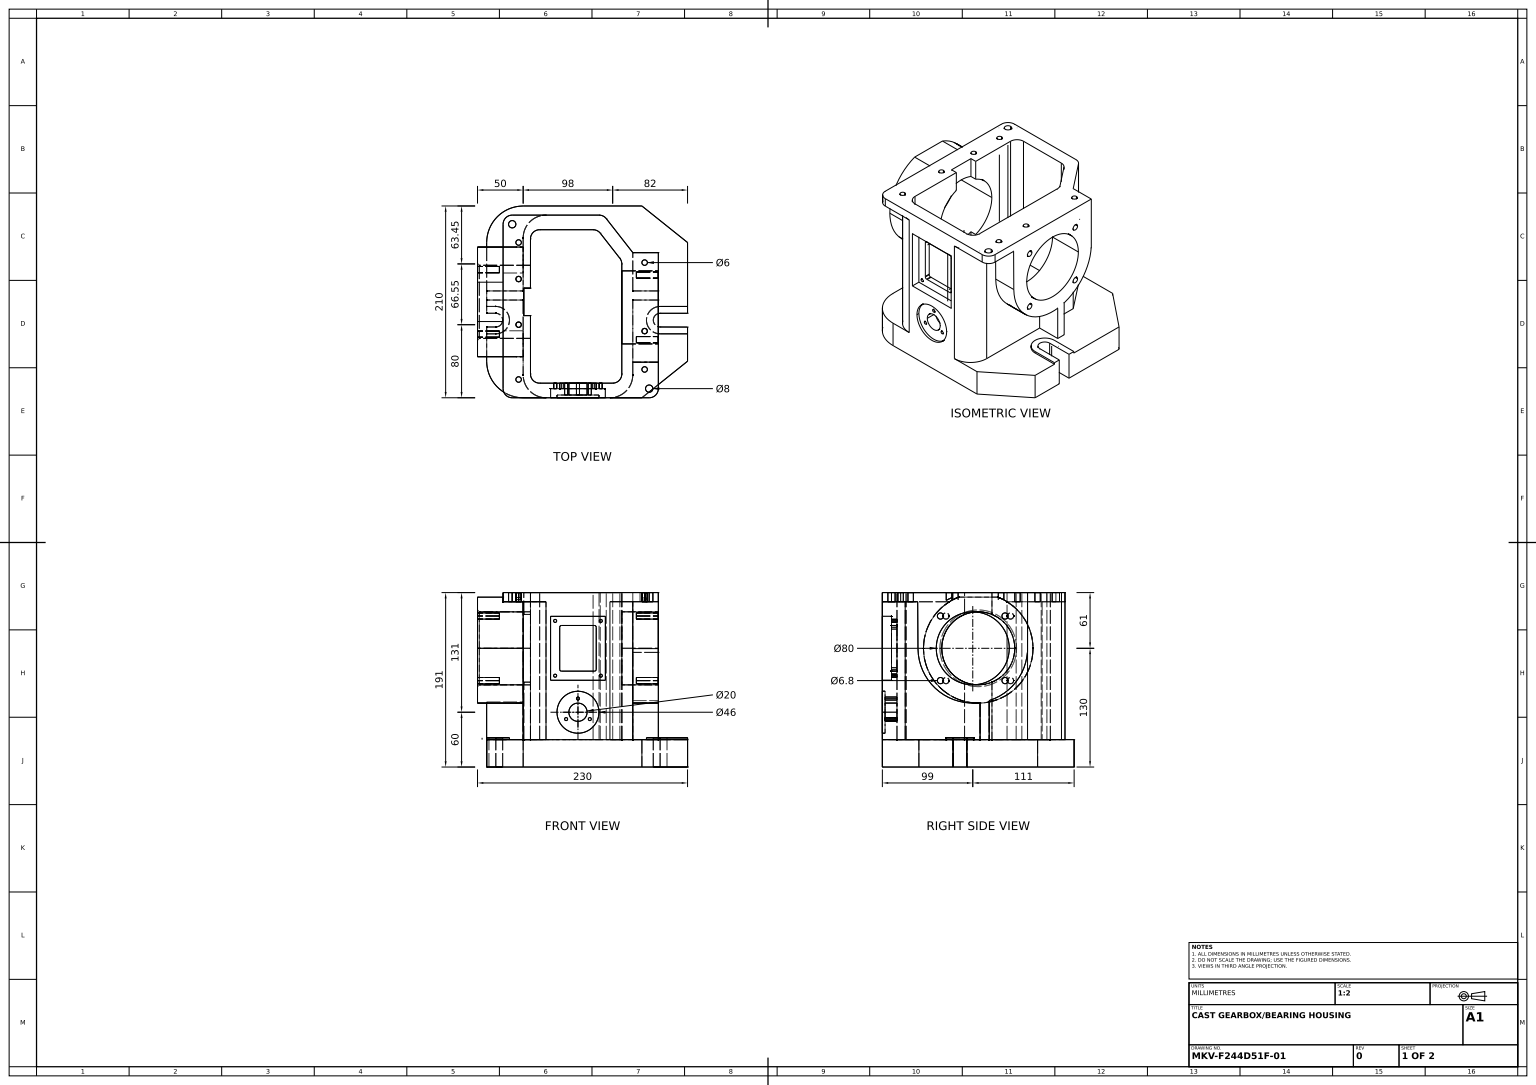
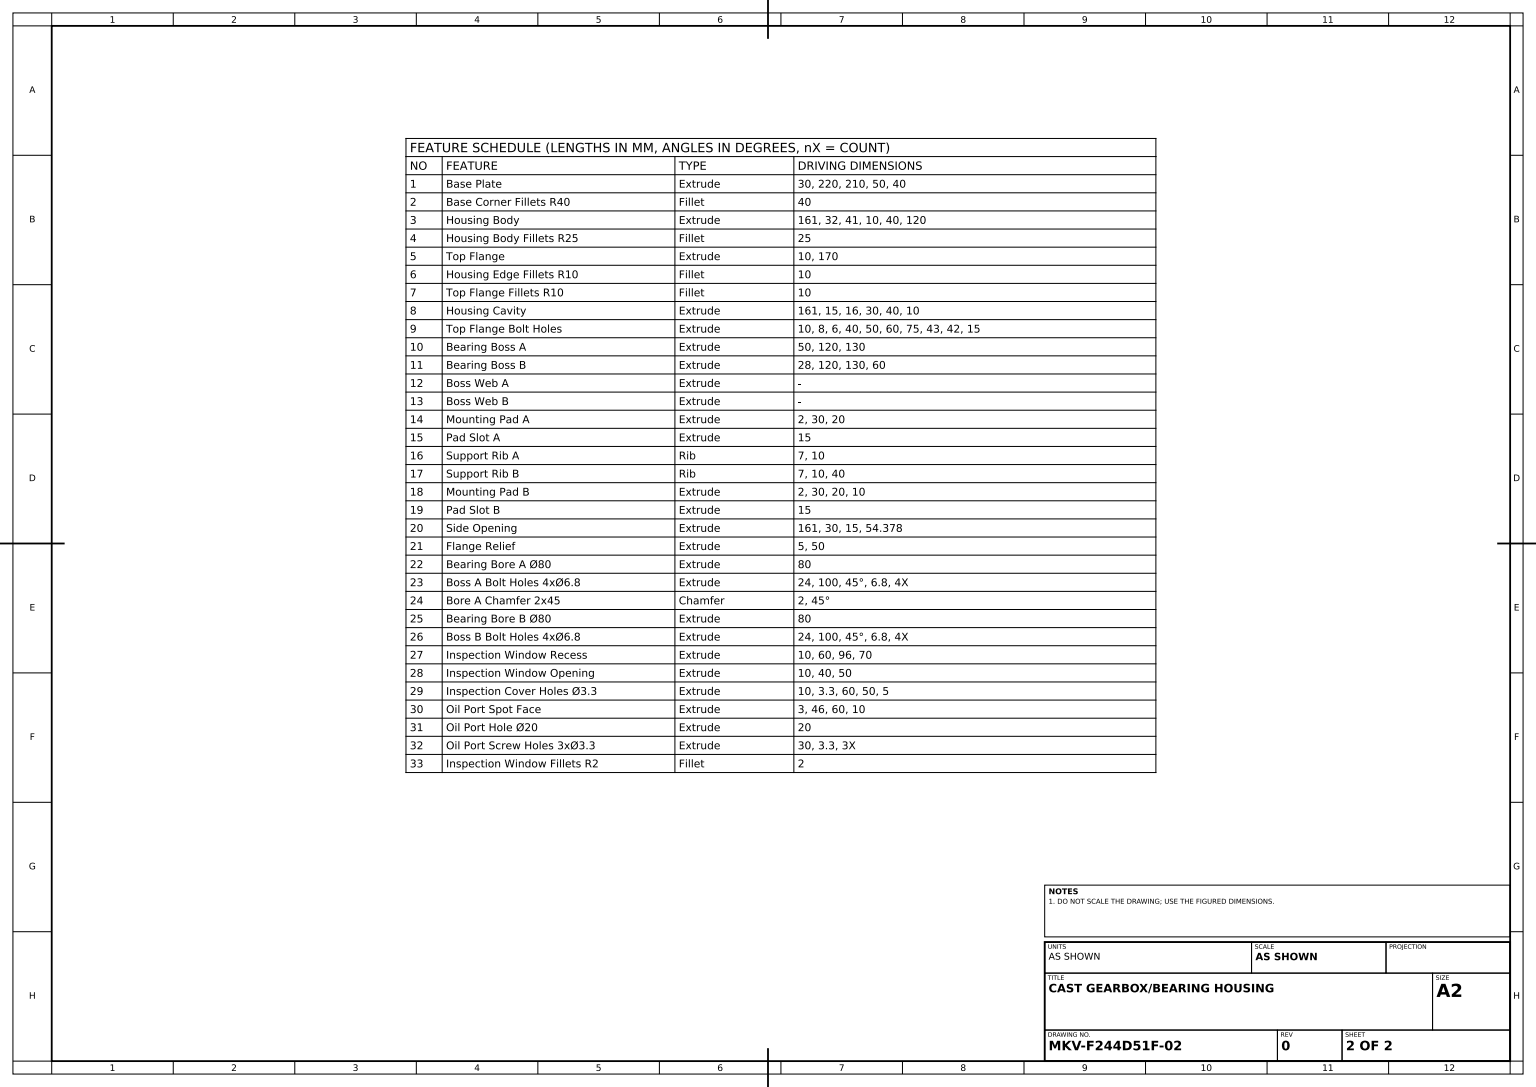
from build123d import *

# Parameters (mm, degrees)
BASE_PLATE_DEPTH                   = 30
BASE_CORNER_FILLETS_R40_R          = 40
HOUSING_BODY_DEPTH                 = 161
HOUSING_BODY_FILLETS_R25_R         = 25
TOP_FLANGE_DEPTH                   = 10
HOUSING_EDGE_FILLETS_R10_R         = 10
TOP_FLANGE_FILLETS_R10_R           = 10
HOUSING_CAVITY_DEPTH               = 161
TOP_FLANGE_BOLT_HOLES_SKETCH_R     = 4
TOP_FLANGE_BOLT_HOLES_SKETCH_R_2   = 3
TOP_FLANGE_BOLT_HOLES_DEPTH        = 10
BEARING_BOSS_A_SKETCH_R            = 60
BEARING_BOSS_A_DEPTH               = 50
BEARING_BOSS_B_SKETCH_R            = 60
BEARING_BOSS_B_DEPTH               = 28
BOSS_WEB_A_REACH                   = 277.975
BOSS_WEB_A_END_RADIUS              = 60
BOSS_WEB_A_SKETCH_W                = 28
BOSS_WEB_A_SKETCH_H                = 55.5
BOSS_WEB_B_REACH                   = 296.466
MOUNTING_PAD_A_DEPTH               = 2
PAD_SLOT_A_DEPTH                   = 226.179928128
SUPPORT_RIB_A_REACH                = 253.843
SUPPORT_RIB_A_SKETCH_WALL_W        = 545.68641053
SUPPORT_RIB_A_SKETCH_WALL_H        = 10
SUPPORT_RIB_B_REACH                = 253.843
SUPPORT_RIB_B_SKETCH_WALL_W        = 545.68641053
SUPPORT_RIB_B_SKETCH_WALL_H        = 10
MOUNTING_PAD_B_DEPTH               = 2
PAD_SLOT_B_DEPTH                   = 226.179928128
SIDE_OPENING_SKETCH_W              = 15
SIDE_OPENING_SKETCH_H              = 30
SIDE_OPENING_DEPTH                 = 161
FLANGE_RELIEF_SKETCH_W             = 28
FLANGE_RELIEF_SKETCH_H             = 50
FLANGE_RELIEF_DEPTH                = 5
BEARING_BORE_A_80_REACH            = 318.869
BEARING_BORE_A_SKETCH_R            = 40
BOSS_A_BOLT_HOLES_SKETCH_R         = 3.4
BOSS_A_BOLT_HOLES_4X_6_8_DEPTH     = 24
BORE_A_CHAMFER_2X45_SIZE           = 2
BEARING_BORE_B_80_REACH            = 296.466
BEARING_BORE_B_SKETCH_R            = 40
BOSS_B_BOLT_HOLES_SKETCH_R         = 3.4
BOSS_B_BOLT_HOLES_4X_6_8_DEPTH     = 24
INSPECTION_WINDOW_RECESS_SKETCH_W  = 60
INSPECTION_WINDOW_RECESS_SKETCH_H  = 70
INSPECTION_WINDOW_RECESS_DEPTH     = 10
INSPECTION_WINDOW_OPENING_SKETCH_W = 40
INSPECTION_WINDOW_OPENING_SKETCH_H = 50
INSPECTION_WINDOW_OPENING_DEPTH    = 10
INSPECTION_COVER_HOLES_SKETCH_R    = 1.65
INSPECTION_COVER_HOLES_3_3_DEPTH   = 10
OIL_PORT_SPOT_FACE_SKETCH_R        = 23
OIL_PORT_SPOT_FACE_DEPTH           = 3
OIL_PORT_HOLE_20_REACH             = 308.154
OIL_PORT_HOLE_SKETCH_R             = 10
OIL_PORT_SCREW_HOLES_3X_3_3_REACH  = 308.154
OIL_PORT_SCREW_HOLES_SKETCH_R      = 1.65
INSPECTION_WINDOW_FILLETS_R2_R     = 2


with BuildPart() as part:
    # Base Plate Sketch → Base Plate (new body)
    with BuildSketch(Plane(origin=(0, 0, 0), x_dir=(1, 0, 0), z_dir=(0, 1, 0))):
        Polygon((60, 105), (110, 65), (110, -65), (60, -105), (-110, -105), (-110, 105), align=None)
    extrude(amount=BASE_PLATE_DEPTH)

    # Base Corner Fillets R40
    base_corner_fillets_r40_edges = [part.edges().sort_by_distance(p)[0] for p in [
        (-110, 15, -105),
        (-110, 15, 105),
    ]]
    fillet(base_corner_fillets_r40_edges, radius=BASE_CORNER_FILLETS_R40_R)

    # Housing Body Sketch → Housing Body (add)
    with BuildSketch(Plane(origin=(0, 30, 0), x_dir=(1, 0, 0), z_dir=(0, 1, 0))):
        Polygon((-70, 95), (18, 95), (50, 54), (50, -105), (-70, -105), align=None)
    extrude(amount=HOUSING_BODY_DEPTH)

    # Housing Body Fillets R25
    housing_body_fillets_r25_edges = [part.edges().sort_by_distance(p)[0] for p in [
        (-70, 110.5, -95),
        (-70, 110.5, 105),
        (50, 110.5, 105),
    ]]
    fillet(housing_body_fillets_r25_edges, radius=HOUSING_BODY_FILLETS_R25_R)

    # Top Flange Sketch → Top Flange (add)
    with BuildSketch(Plane(origin=(0, 191, 0), x_dir=(1, 0, 0), z_dir=(0, 1, 0))):
        Polygon((18, 95), (-92, 95), (-92, -105), (78, -105), (78, 54), (50, 54), align=None)
    extrude(amount=-TOP_FLANGE_DEPTH)

    # Housing Edge Fillets R10
    housing_edge_fillets_r10_edges = [part.edges().sort_by_distance(p)[0] for p in [
        (18, 110.5, -95),
    ]]
    fillet(housing_edge_fillets_r10_edges, radius=HOUSING_EDGE_FILLETS_R10_R)

    # Top Flange Fillets R10
    top_flange_fillets_r10_edges = [part.edges().sort_by_distance(p)[0] for p in [
        (-92, 186, -95),
        (78, 186, 105),
        (-92, 186, 105),
    ]]
    fillet(top_flange_fillets_r10_edges, radius=TOP_FLANGE_FILLETS_R10_R)

    # Housing Cavity Sketch → Housing Cavity (cut)
    with BuildSketch(Plane(origin=(0, 191, 0), x_dir=(1, 0, 0), z_dir=(0, 1, 0))):
        with BuildLine():
            Line((35.883157835, 47.707697229), (14.462661191, 75.152708554))
            ThreePointArc((14.462661191, 75.152708554), (10.965441936, 77.986853886), (6.579503356, 79))
            Line((6.579503356, 79), (-52, 79))
            ThreePointArc((-52, 79), (-59.071067812, 76.071067812), (-62, 69))
            Line((-62, 69), (-62, -79))
            ThreePointArc((-62, -79), (-59.071067812, -86.071067812), (-52, -89))
            Line((-52, -89), (28, -89))
            ThreePointArc((28, -89), (35.071067812, -86.071067812), (38, -79))
            Line((38, -79), (38, 41.554988675))
            ThreePointArc((38, 41.554988675), (37.455992236, 44.808327088), (35.883157835, 47.707697229))
        make_face()
    extrude(amount=-HOUSING_CAVITY_DEPTH, mode=Mode.SUBTRACT)

    # Top Flange Bolt Holes Sketch → Top Flange Bolt Holes (cut)
    with BuildSketch(Plane(origin=(0, 191, 0), x_dir=(1, 0, 0), z_dir=(0, 1, 0))):
        with Locations(Location((-82, 85, 0), (0, 0, 270))):
            Circle(TOP_FLANGE_BOLT_HOLES_SKETCH_R)
        with Locations(Location((68, -95, 0), (0, 0, 270))):
            Circle(TOP_FLANGE_BOLT_HOLES_SKETCH_R)
        with Locations(Location((-75, 65, 0), (0, 0, 270))):
            Circle(TOP_FLANGE_BOLT_HOLES_SKETCH_R_2)
        with Locations(Location((-75, 25, 0), (0, 0, 270))):
            Circle(TOP_FLANGE_BOLT_HOLES_SKETCH_R_2)
        with Locations(Location((-75, -25, 0), (0, 0, 270))):
            Circle(TOP_FLANGE_BOLT_HOLES_SKETCH_R_2)
        with Locations(Location((-75, -85, 0), (0, 0, 270))):
            Circle(TOP_FLANGE_BOLT_HOLES_SKETCH_R_2)
        with Locations(Location((63, 43, 0), (0, 0, 270))):
            Circle(TOP_FLANGE_BOLT_HOLES_SKETCH_R_2)
        with Locations(Location((63, -32, 0), (0, 0, 270))):
            Circle(TOP_FLANGE_BOLT_HOLES_SKETCH_R_2)
        with Locations(Location((63, -74, 0), (0, 0, 270))):
            Circle(TOP_FLANGE_BOLT_HOLES_SKETCH_R_2)
    extrude(amount=-TOP_FLANGE_BOLT_HOLES_DEPTH, mode=Mode.SUBTRACT)

    # Bearing Boss A Sketch → Bearing Boss A (add)
    with BuildSketch(Plane.ZY.offset(70)):
        with Locations(Location((0, 130, 0), (0, 0, 121.788330617))):
            Circle(BEARING_BOSS_A_SKETCH_R)
    extrude(amount=BEARING_BOSS_A_DEPTH)

    # Bearing Boss B Sketch → Bearing Boss B (add)
    with BuildSketch(Plane(origin=(50, 0, 0), x_dir=(0, 0, -1), z_dir=(1, 0, 0))):
        with Locations((-6, 130)):
            Circle(BEARING_BOSS_B_SKETCH_R)
    extrude(amount=BEARING_BOSS_B_DEPTH)

    # Boss Web A: up to this cylinder (the profile starts outside it)
    boss_web_a_end = Plane(origin=(64, 130, 6), z_dir=(-1, 0, 0)) * Cylinder(BOSS_WEB_A_END_RADIUS, 676.95, mode=Mode.PRIVATE)
    # Boss Web A Sketch → Boss Web A (add, up to the surface)
    with BuildSketch(Plane(origin=(0, 0, -54), x_dir=(-1, 0, 0), z_dir=(0, 0, -1)), mode=Mode.PRIVATE) as boss_web_a_sk1:
        with Locations((-64, 153.25)):
            Rectangle(BOSS_WEB_A_SKETCH_W, BOSS_WEB_A_SKETCH_H)
    boss_web_a_tool1 = extrude(boss_web_a_sk1.sketch, amount=-BOSS_WEB_A_REACH, mode=Mode.PRIVATE) - boss_web_a_end
    add(boss_web_a_tool1.solids().sort_by_distance((64, 153.25, -54))[0])
    add(boss_web_a_tool1.solids().sort_by_distance((64, 153.25, -54))[1])

    # Boss Web B Sketch → Boss Web B (add, up to next)
    with BuildSketch(Plane(origin=(78, 0, 0), x_dir=(0, 0, -1), z_dir=(1, 0, 0)), mode=Mode.PRIVATE) as boss_web_b_sk1:
        with BuildLine():
            Line((-65.998945111, 129.644211289), (-66.303480629, 181))
            Line((-66.303480629, 181), (-37.606961259, 181))
            ThreePointArc((-37.606961259, 181), (-58.509663672, 159.029902188), (-65.998945111, 129.644211289))
        make_face()
    boss_web_b_tool1 = extrude(boss_web_b_sk1.sketch, amount=-BOSS_WEB_B_REACH, mode=Mode.PRIVATE) - part.part
    add(boss_web_b_tool1.solids().sort_by_distance((78, 168.840925, 58.135021))[0])

    # Mounting Pad A Sketch → Mounting Pad A (add)
    with BuildSketch(Plane(origin=(0, 30, 0), x_dir=(1, 0, 0), z_dir=(0, 1, 0))):
        with BuildLine():
            Line((80, -5), (110, -5))
            Line((110, -5), (110, -35))
            Line((110, -35), (80, -35))
            ThreePointArc((80, -35), (65, -20), (80, -5))
        make_face()
    extrude(amount=MOUNTING_PAD_A_DEPTH)

    # Pad Slot A Sketch → Pad Slot A (cut, through all)
    with BuildSketch(Plane(origin=(0, 32, 0), x_dir=(1, 0, 0), z_dir=(0, 1, 0))):
        with BuildLine():
            Line((80, -12.5), (110, -12.5))
            Line((110, -12.5), (110, -27.596191178))
            Line((110, -27.596191178), (79.975961959, -27.499961478))
            ThreePointArc((79.975961959, -27.499961478), (72.50000963, -19.987980964), (80, -12.5))
        make_face()
    extrude(amount=-PAD_SLOT_A_DEPTH, mode=Mode.SUBTRACT)

    # Support Rib A Sketch wall → Support Rib A (add, up to next)
    with BuildSketch(Plane(origin=(78, 50, -7), x_dir=(0, -1, 0), z_dir=(1, 0, 0)), mode=Mode.PRIVATE) as support_rib_a_sk1:
        Rectangle(SUPPORT_RIB_A_SKETCH_WALL_W, SUPPORT_RIB_A_SKETCH_WALL_H)
    support_rib_a_tool1 = extrude(support_rib_a_sk1.sketch, amount=-SUPPORT_RIB_A_REACH, mode=Mode.PRIVATE) - part.part
    add(support_rib_a_tool1.solids().sort_by_distance((78, 50, -7))[0])

    # Support Rib B Sketch wall → Support Rib B (add, up to next)
    with BuildSketch(Plane(origin=(-110, 50, -7), x_dir=(0, -1, 0), z_dir=(1, 0, 0)), mode=Mode.PRIVATE) as support_rib_b_sk1:
        Rectangle(SUPPORT_RIB_B_SKETCH_WALL_W, SUPPORT_RIB_B_SKETCH_WALL_H)
    support_rib_b_tool1 = extrude(support_rib_b_sk1.sketch, amount=SUPPORT_RIB_B_REACH, mode=Mode.PRIVATE) - part.part
    add(support_rib_b_tool1.solids().sort_by_distance((-110, 50, -7))[0])

    # Mounting Pad B Sketch → Mounting Pad B (add)
    with BuildSketch(Plane(origin=(0, 30, 0), x_dir=(1, 0, 0), z_dir=(0, 1, 0))):
        with BuildLine():
            Line((-100, -5), (-110, -5))
            Line((-110, -5), (-110, -35))
            Line((-110, -35), (-100, -35))
            ThreePointArc((-100, -35), (-85, -20), (-100, -5))
        make_face()
    extrude(amount=MOUNTING_PAD_B_DEPTH)

    # Pad Slot B Sketch → Pad Slot B (cut, through all)
    with BuildSketch(Plane(origin=(0, 32, 0), x_dir=(1, 0, 0), z_dir=(0, 1, 0))):
        with BuildLine():
            Line((-100, -12.5), (-110, -12.5))
            Line((-110, -12.5), (-110, -27.5))
            Line((-110, -27.5), (-100, -27.5))
            ThreePointArc((-100, -27.5), (-92.5, -20), (-100, -12.5))
        make_face()
    extrude(amount=-PAD_SLOT_B_DEPTH, mode=Mode.SUBTRACT)

    # Side Opening Sketch → Side Opening (cut)
    with BuildSketch(Plane(origin=(0, 191, 0), x_dir=(1, 0, 0), z_dir=(0, 1, 0))):
        with Locations((-61.877981693, 0)):
            Rectangle(SIDE_OPENING_SKETCH_W, SIDE_OPENING_SKETCH_H)
    extrude(amount=-SIDE_OPENING_DEPTH, mode=Mode.SUBTRACT)

    # Flange Relief Sketch → Flange Relief (cut)
    with BuildSketch(Plane(origin=(0, 191, 0), x_dir=(1, 0, 0), z_dir=(0, 1, 0))):
        with Locations((-106, 0)):
            Rectangle(FLANGE_RELIEF_SKETCH_W, FLANGE_RELIEF_SKETCH_H)
    extrude(amount=-FLANGE_RELIEF_DEPTH, mode=Mode.SUBTRACT)

    # Bearing Bore A Sketch → Bearing Bore A Ø80 (cut, up to next)
    with BuildSketch(Plane.ZY.offset(120), mode=Mode.PRIVATE) as bearing_bore_a_80_sk1:
        with Locations((0, 130)):
            Circle(BEARING_BORE_A_SKETCH_R)
    bearing_bore_a_80_tool1 = extrude(bearing_bore_a_80_sk1.sketch, amount=-BEARING_BORE_A_80_REACH, mode=Mode.PRIVATE) & part.part
    add(bearing_bore_a_80_tool1.solids().sort_by_distance((-120, 130, 0))[0], mode=Mode.SUBTRACT)

    # Boss A Bolt Holes Sketch → Boss A Bolt Holes 4xØ6.8 (cut)
    with BuildSketch(Plane.ZY.offset(120)):
        with Locations((35.355339059, 94.644660941)):
            Circle(BOSS_A_BOLT_HOLES_SKETCH_R)
        with Locations((-35.355339059, 94.644660941)):
            Circle(BOSS_A_BOLT_HOLES_SKETCH_R)
        with Locations((-35.355339059, 165.355339059)):
            Circle(BOSS_A_BOLT_HOLES_SKETCH_R)
        with Locations((35.355339059, 165.355339059)):
            Circle(BOSS_A_BOLT_HOLES_SKETCH_R)
    extrude(amount=-BOSS_A_BOLT_HOLES_4X_6_8_DEPTH, mode=Mode.SUBTRACT)

    # Bore A Chamfer 2x45
    bore_a_chamfer_2x45_edges = [part.edges().sort_by_distance(p)[0] for p in [
        (-120, 130, -40),
    ]]
    chamfer(bore_a_chamfer_2x45_edges, length=BORE_A_CHAMFER_2X45_SIZE)

    # Bearing Bore B Sketch → Bearing Bore B Ø80 (cut, up to next)
    with BuildSketch(Plane(origin=(78, 0, 0), x_dir=(0, 0, -1), z_dir=(1, 0, 0)), mode=Mode.PRIVATE) as bearing_bore_b_80_sk1:
        with Locations((-6, 130)):
            Circle(BEARING_BORE_B_SKETCH_R)
    bearing_bore_b_80_tool1 = extrude(bearing_bore_b_80_sk1.sketch, amount=-BEARING_BORE_B_80_REACH, mode=Mode.PRIVATE) & part.part
    add(bearing_bore_b_80_tool1.solids().sort_by_distance((78, 130, 6))[0], mode=Mode.SUBTRACT)

    # Boss B Bolt Holes Sketch → Boss B Bolt Holes 4xØ6.8 (cut)
    with BuildSketch(Plane(origin=(78, 0, 0), x_dir=(0, 0, -1), z_dir=(1, 0, 0))):
        with Locations((29.355339059, 94.644660941)):
            Circle(BOSS_B_BOLT_HOLES_SKETCH_R)
        with Locations((-41.355339059, 94.644660941)):
            Circle(BOSS_B_BOLT_HOLES_SKETCH_R)
        with Locations((-41.355339059, 165.355339059)):
            Circle(BOSS_B_BOLT_HOLES_SKETCH_R)
        with Locations((29.355339059, 165.355339059)):
            Circle(BOSS_B_BOLT_HOLES_SKETCH_R)
    extrude(amount=-BOSS_B_BOLT_HOLES_4X_6_8_DEPTH, mode=Mode.SUBTRACT)

    # Inspection Window Recess Sketch → Inspection Window Recess (cut)
    with BuildSketch(Plane.XY.offset(105)):
        with Locations((-10, 130)):
            Rectangle(INSPECTION_WINDOW_RECESS_SKETCH_W, INSPECTION_WINDOW_RECESS_SKETCH_H)
    extrude(amount=-INSPECTION_WINDOW_RECESS_DEPTH, mode=Mode.SUBTRACT)

    # Inspection Window Opening Sketch → Inspection Window Opening (cut)
    with BuildSketch(Plane.XY.offset(95)):
        with Locations((-10, 130)):
            Rectangle(INSPECTION_WINDOW_OPENING_SKETCH_W, INSPECTION_WINDOW_OPENING_SKETCH_H)
    extrude(amount=-INSPECTION_WINDOW_OPENING_DEPTH, mode=Mode.SUBTRACT)

    # Inspection Cover Holes Sketch → Inspection Cover Holes Ø3.3 (cut)
    with BuildSketch(Plane.XY.offset(95)):
        with Locations((-35, 160)):
            Circle(INSPECTION_COVER_HOLES_SKETCH_R)
        with Locations((15, 160)):
            Circle(INSPECTION_COVER_HOLES_SKETCH_R)
        with Locations((-35, 100)):
            Circle(INSPECTION_COVER_HOLES_SKETCH_R)
        with Locations((15, 100)):
            Circle(INSPECTION_COVER_HOLES_SKETCH_R)
    extrude(amount=-INSPECTION_COVER_HOLES_3_3_DEPTH, mode=Mode.SUBTRACT)

    # Oil Port Spot Face Sketch → Oil Port Spot Face (cut)
    with BuildSketch(Plane.XY.offset(105)):
        with Locations((-10, 60)):
            Circle(OIL_PORT_SPOT_FACE_SKETCH_R)
    extrude(amount=-OIL_PORT_SPOT_FACE_DEPTH, mode=Mode.SUBTRACT)

    # Oil Port Hole Sketch → Oil Port Hole Ø20 (cut, up to next)
    with BuildSketch(Plane.XY.offset(102), mode=Mode.PRIVATE) as oil_port_hole_20_sk1:
        with Locations((-10, 60)):
            Circle(OIL_PORT_HOLE_SKETCH_R)
    oil_port_hole_20_tool1 = extrude(oil_port_hole_20_sk1.sketch, amount=-OIL_PORT_HOLE_20_REACH, mode=Mode.PRIVATE) & part.part
    add(oil_port_hole_20_tool1.solids().sort_by_distance((-10, 60, 102))[0], mode=Mode.SUBTRACT)

    # Oil Port Screw Holes Sketch → Oil Port Screw Holes 3xØ3.3 (cut, up to next)
    with BuildSketch(Plane.XY.offset(102), mode=Mode.PRIVATE) as oil_port_screw_holes_3x_3_3_sk1:
        with Locations((-10, 75)):
            Circle(OIL_PORT_SCREW_HOLES_SKETCH_R)
    oil_port_screw_holes_3x_3_3_tool1 = extrude(oil_port_screw_holes_3x_3_3_sk1.sketch, amount=-OIL_PORT_SCREW_HOLES_3X_3_3_REACH, mode=Mode.PRIVATE) & part.part
    # Oil Port Screw Holes Sketch → Oil Port Screw Holes 3xØ3.3 (cut, up to next)
    with BuildSketch(Plane.XY.offset(102), mode=Mode.PRIVATE) as oil_port_screw_holes_3x_3_3_sk2:
        with Locations((2.990381057, 52.5)):
            Circle(OIL_PORT_SCREW_HOLES_SKETCH_R)
    oil_port_screw_holes_3x_3_3_tool2 = extrude(oil_port_screw_holes_3x_3_3_sk2.sketch, amount=-OIL_PORT_SCREW_HOLES_3X_3_3_REACH, mode=Mode.PRIVATE) & part.part
    # Oil Port Screw Holes Sketch → Oil Port Screw Holes 3xØ3.3 (cut, up to next)
    with BuildSketch(Plane.XY.offset(102), mode=Mode.PRIVATE) as oil_port_screw_holes_3x_3_3_sk3:
        with Locations((-22.990381057, 52.5)):
            Circle(OIL_PORT_SCREW_HOLES_SKETCH_R)
    oil_port_screw_holes_3x_3_3_tool3 = extrude(oil_port_screw_holes_3x_3_3_sk3.sketch, amount=-OIL_PORT_SCREW_HOLES_3X_3_3_REACH, mode=Mode.PRIVATE) & part.part
    add(oil_port_screw_holes_3x_3_3_tool1.solids().sort_by_distance((-10, 75, 102))[0], mode=Mode.SUBTRACT)
    add(oil_port_screw_holes_3x_3_3_tool2.solids().sort_by_distance((2.990381, 52.5, 102))[0], mode=Mode.SUBTRACT)
    add(oil_port_screw_holes_3x_3_3_tool3.solids().sort_by_distance((-22.990381, 52.5, 102))[0], mode=Mode.SUBTRACT)

    # Inspection Window Fillets R2
    inspection_window_fillets_r2_edges = [part.edges().sort_by_distance(p)[0] for p in [
        (10, 155, 92),
        (10, 105, 92),
        (-30, 105, 92),
        (-30, 155, 92),
    ]]
    fillet(inspection_window_fillets_r2_edges, radius=INSPECTION_WINDOW_FILLETS_R2_R)


solid = part.part
